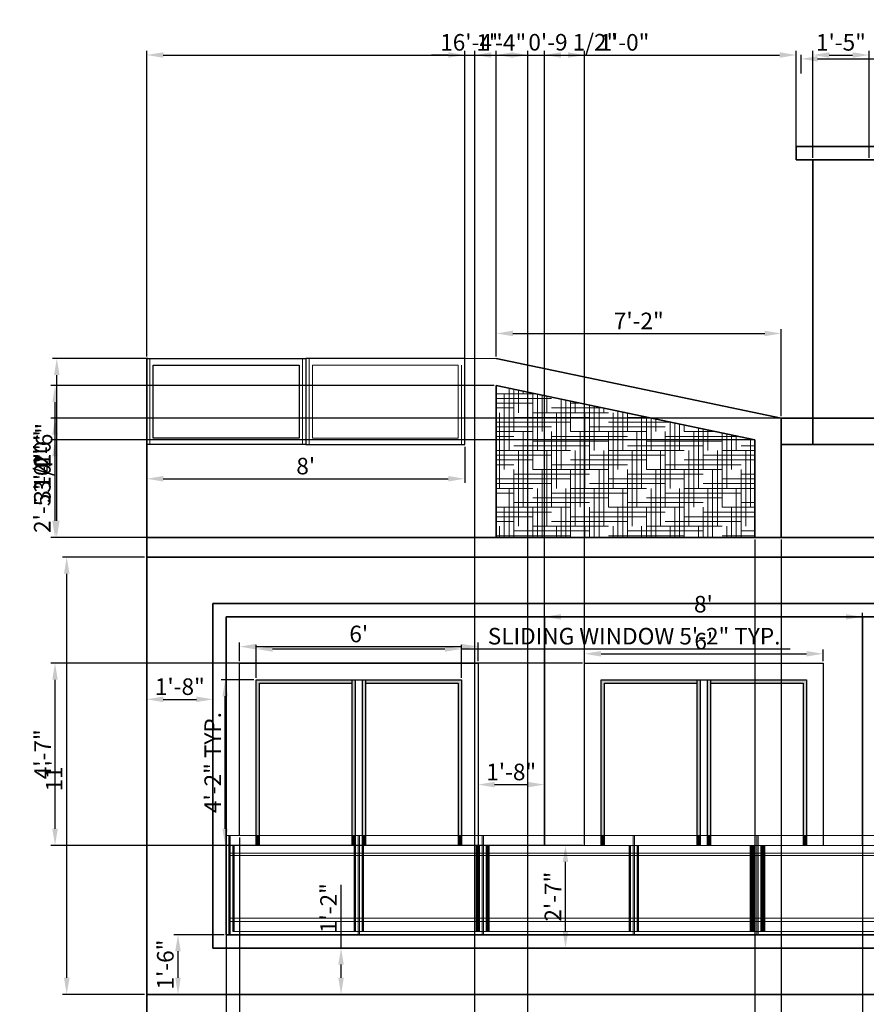
# Model space of a CAD drawing. Units: inches. Extents: x 2406 to 2953, y 1777 to 2285.
# Tile 2 of 5: x 2406 to 2661, y 1987 to 2285. Entities that reach past the tile are written whole.
import ezdxf

# ---------------------------------------------------------------- set-up
doc = ezdxf.new("R2010")
doc.units = ezdxf.units.IN
for name, color, linetype, lineweight in [('A-ANNO-DIMS', 2, 'Continuous', 18), ('A-ELEV', 7, 'Continuous', 35), ('A-ELEV-PATT', 253, 'Continuous', 13), ('A-FLOR-HRAL', 6, 'Continuous', 18), ('A-GLAZ', 4, 'Continuous', 25)]:
    doc.layers.add(name, color=color, linetype=linetype, lineweight=lineweight)
doc.styles.get("Standard").update_dxf_attribs({"font": 'arial.ttf'})
doc.dimstyles.new('ISO-25', dxfattribs={"dimtxt": 5, "dimasz": 5, "dimexe": 1.25, "dimexo": 0.625, "dimtad": 1, "dimdec": 0, "dimlunit": 3, "dimtxsty": 'Standard', "dimcen": 2.5, "dimadec": 0, "dimazin": 0, "dimtfac": 1, "dimtdec": 0, "dimtmove": 0, "dimatfit": 3, "dimfxl": 1, "dimarcsym": 0})

# ---------------------------------------------------------------- blocks, each defined once
blk = doc.blocks.new('*D7')
at = {"layer": 'A-ANNO-DIMS', "color": 0, "lineweight": -2, "transparency": 16777216}
for p, q in [((2443.21, 2122.34), (2418.45, 2122.34)), ((2419.7, 1995.34), (2419.7, 2117.34)), ((2443.21, 1990.34), (2418.45, 1990.34))]:
    blk.add_line(p, q, dxfattribs=at)
at = {"layer": 'A-ANNO-DIMS', "color": 0, "transparency": 16777216}
for points in [[(2418.87, 2117.34), (2420.53, 2117.34), (2419.7, 2122.34)], [(2418.87, 1995.34), (2420.53, 1995.34), (2419.7, 1990.34)]]:
    blk.add_solid(points, dxfattribs=at)
at = {"layer": 'Defpoints', "color": 0, "transparency": 16777216}
for p in [(2419.7, 2122.34), (2443.83, 2122.34), (2443.83, 1990.34)]:
    blk.add_point(p, dxfattribs=at)
at = {"layer": 'A-ANNO-DIMS', "color": 0, "transparency": 16777216, "insert": (2416.57, 2056.34), "char_height": 5, "attachment_point": 5, "rotation": 90}
blk.add_mtext("11'", dxfattribs=at)
blk = doc.blocks.new('*D8')
at = {"layer": 'A-ANNO-DIMS', "color": 0, "lineweight": -2, "transparency": 16777216}
for p, q in [((2444.21, 2182.34), (2415.46, 2182.34)), ((2416.71, 2133.34), (2416.71, 2177.34)), ((2443.21, 2128.34), (2415.46, 2128.34))]:
    blk.add_line(p, q, dxfattribs=at)
at = {"layer": 'A-ANNO-DIMS', "color": 0, "transparency": 16777216}
for points in [[(2415.88, 2177.34), (2417.55, 2177.34), (2416.71, 2182.34)], [(2415.88, 2133.34), (2417.55, 2133.34), (2416.71, 2128.34)]]:
    blk.add_solid(points, dxfattribs=at)
at = {"layer": 'Defpoints', "color": 0, "transparency": 16777216}
for p in [(2416.71, 2182.34), (2444.83, 2182.34), (2443.83, 2128.34)]:
    blk.add_point(p, dxfattribs=at)
at = {"layer": 'A-ANNO-DIMS', "color": 0, "transparency": 16777216, "insert": (2413.53, 2155.34), "char_height": 5, "attachment_point": 5, "rotation": 90}
blk.add_mtext('4\'-6"', dxfattribs=at)
blk = doc.blocks.new('*D9')
at = {"layer": 'A-ANNO-DIMS', "color": 0, "lineweight": -2, "transparency": 16777216}
for p, q in [((2549.33, 2182.97), (2549.33, 2191.16)), ((2554.33, 2189.91), (2630.33, 2189.91)), ((2635.33, 2164.97), (2635.33, 2191.16))]:
    blk.add_line(p, q, dxfattribs=at)
at = {"layer": 'A-ANNO-DIMS', "color": 0, "transparency": 16777216}
for points in [[(2554.33, 2190.74), (2554.33, 2189.08), (2549.33, 2189.91)], [(2630.33, 2190.74), (2630.33, 2189.08), (2635.33, 2189.91)]]:
    blk.add_solid(points, dxfattribs=at)
at = {"layer": 'Defpoints', "color": 0, "transparency": 16777216}
for p in [(2635.33, 2189.91), (2549.33, 2182.34), (2635.33, 2164.34)]:
    blk.add_point(p, dxfattribs=at)
at = {"layer": 'A-ANNO-DIMS', "color": 0, "transparency": 16777216, "insert": (2592.33, 2193.05), "char_height": 5, "attachment_point": 5}
blk.add_mtext('7\'-2"', dxfattribs=at)
blk = doc.blocks.new('*D10')
at = {"layer": 'A-ANNO-DIMS', "color": 0, "lineweight": -2, "transparency": 16777216}
for p, q in [((2641.3, 2268.37), (2641.3, 2274.08)), ((2646.3, 2272.83), (2830.3, 2272.83)), ((2835.3, 2268.37), (2835.3, 2274.08))]:
    blk.add_line(p, q, dxfattribs=at)
at = {"layer": 'A-ANNO-DIMS', "color": 0, "transparency": 16777216}
for points in [[(2646.3, 2273.66), (2646.3, 2272), (2641.3, 2272.83)], [(2830.3, 2273.66), (2830.3, 2272), (2835.3, 2272.83)]]:
    blk.add_solid(points, dxfattribs=at)
at = {"layer": 'Defpoints', "color": 0, "transparency": 16777216}
for p in [(2835.3, 2272.83), (2641.3, 2267.75), (2835.3, 2267.75)]:
    blk.add_point(p, dxfattribs=at)
at = {"layer": 'A-ANNO-DIMS', "color": 0, "transparency": 16777216, "insert": (2738.3, 2276.01), "char_height": 5, "attachment_point": 5}
blk.add_mtext('16\'-2"', dxfattribs=at)
blk = doc.blocks.new('*D13')
at = {"layer": 'A-ANNO-DIMS', "color": 0, "lineweight": -2, "transparency": 16777216}
for p, q in [((2563.83, 2097.76), (2563.83, 2105.59)), ((2659.83, 2099.01), (2659.83, 2105.59)), ((2568.83, 2104.34), (2654.83, 2104.34))]:
    blk.add_line(p, q, dxfattribs=at)
at = {"layer": 'A-ANNO-DIMS', "color": 0, "transparency": 16777216}
for points in [[(2568.83, 2105.17), (2568.83, 2103.51), (2563.83, 2104.34)], [(2654.83, 2105.17), (2654.83, 2103.51), (2659.83, 2104.34)]]:
    blk.add_solid(points, dxfattribs=at)
at = {"layer": 'Defpoints', "color": 0, "transparency": 16777216}
for p in [(2659.83, 2104.34), (2563.83, 2097.13), (2659.83, 2098.38)]:
    blk.add_point(p, dxfattribs=at)
at = {"layer": 'A-ANNO-DIMS', "color": 0, "transparency": 16777216, "insert": (2611.83, 2107.52), "char_height": 5, "attachment_point": 5}
blk.add_mtext("8'", dxfattribs=at)
blk = doc.blocks.new('*D14')
at = {"layer": 'A-ANNO-DIMS', "color": 0, "lineweight": -2, "transparency": 16777216}
for p, q in [((2575.95, 2090.97), (2575.95, 2094.44)), ((2580.95, 2093.19), (2642.95, 2093.19)), ((2647.95, 2090.97), (2647.95, 2094.44))]:
    blk.add_line(p, q, dxfattribs=at)
at = {"layer": 'A-ANNO-DIMS', "color": 0, "transparency": 16777216}
for points in [[(2580.95, 2094.02), (2580.95, 2092.35), (2575.95, 2093.19)], [(2642.95, 2094.02), (2642.95, 2092.35), (2647.95, 2093.19)]]:
    blk.add_solid(points, dxfattribs=at)
at = {"layer": 'Defpoints', "color": 0, "transparency": 16777216}
for p in [(2647.95, 2093.19), (2575.95, 2090.34), (2647.95, 2090.34)]:
    blk.add_point(p, dxfattribs=at)
at = {"layer": 'A-ANNO-DIMS', "color": 0, "transparency": 16777216, "insert": (2611.95, 2096.36), "char_height": 5, "attachment_point": 5}
blk.add_mtext("6'", dxfattribs=at)
blk = doc.blocks.new('*D22')
at = {"layer": 'A-ANNO-DIMS', "color": 0, "lineweight": -2, "transparency": 16777216}
for p, q in [((2467.21, 2008.34), (2452.04, 2008.34)), ((2453.29, 1995.34), (2453.29, 2003.34)), ((2465.03, 1990.34), (2452.04, 1990.34))]:
    blk.add_line(p, q, dxfattribs=at)
at = {"layer": 'A-ANNO-DIMS', "color": 0, "transparency": 16777216}
for points in [[(2452.45, 2003.34), (2454.12, 2003.34), (2453.29, 2008.34)], [(2452.45, 1995.34), (2454.12, 1995.34), (2453.29, 1990.34)]]:
    blk.add_solid(points, dxfattribs=at)
at = {"layer": 'Defpoints', "color": 0, "transparency": 16777216}
for p in [(2453.29, 2008.34), (2467.83, 2008.34), (2465.66, 1990.34)]:
    blk.add_point(p, dxfattribs=at)
at = {"layer": 'A-ANNO-DIMS', "color": 0, "transparency": 16777216, "insert": (2450.11, 1999.34), "char_height": 5, "attachment_point": 5, "rotation": 90}
blk.add_mtext('1\'-6"', dxfattribs=at)
blk = doc.blocks.new('*D23')
at = {"layer": 'A-ANNO-DIMS', "color": 0, "lineweight": -2, "transparency": 16777216}
for p, q in [((2502.49, 2004.34), (2502.49, 2023.41)), ((2496.37, 2004.34), (2503.74, 2004.34)), ((2502.49, 1995.34), (2502.49, 1999.34)), ((2496.37, 1990.34), (2503.74, 1990.34))]:
    blk.add_line(p, q, dxfattribs=at)
at = {"layer": 'A-ANNO-DIMS', "color": 0, "transparency": 16777216}
for points in [[(2501.66, 1999.34), (2503.32, 1999.34), (2502.49, 2004.34)], [(2501.66, 1995.34), (2503.32, 1995.34), (2502.49, 1990.34)]]:
    blk.add_solid(points, dxfattribs=at)
at = {"layer": 'Defpoints', "color": 0, "transparency": 16777216}
for p in [(2495.74, 2004.34), (2502.49, 2004.34), (2495.74, 1990.34)]:
    blk.add_point(p, dxfattribs=at)
at = {"layer": 'A-ANNO-DIMS', "color": 0, "transparency": 16777216, "insert": (2499.36, 2016.38), "char_height": 5, "attachment_point": 5, "rotation": 90}
blk.add_mtext('1\'-2"', dxfattribs=at)
blk = doc.blocks.new('*D24')
at = {"layer": 'A-ANNO-DIMS', "color": 0, "lineweight": -2, "transparency": 16777216}
for p, q in [((2443.83, 2067.83), (2443.83, 2080.68)), ((2448.83, 2079.43), (2458.83, 2079.43)), ((2463.83, 2067.83), (2463.83, 2080.68))]:
    blk.add_line(p, q, dxfattribs=at)
at = {"layer": 'A-ANNO-DIMS', "color": 0, "transparency": 16777216}
for points in [[(2448.83, 2080.27), (2448.83, 2078.6), (2443.83, 2079.43)], [(2458.83, 2080.27), (2458.83, 2078.6), (2463.83, 2079.43)]]:
    blk.add_solid(points, dxfattribs=at)
at = {"layer": 'Defpoints', "color": 0, "transparency": 16777216}
for p in [(2463.83, 2079.43), (2443.83, 2067.21), (2463.83, 2067.21)]:
    blk.add_point(p, dxfattribs=at)
at = {"layer": 'A-ANNO-DIMS', "color": 0, "transparency": 16777216, "insert": (2453.83, 2082.61), "char_height": 5, "attachment_point": 5}
blk.add_mtext('1\'-8"', dxfattribs=at)
blk = doc.blocks.new('*D33')
at = {"layer": 'A-ANNO-DIMS', "color": 0, "lineweight": -2, "transparency": 16777216}
for p, q in [((2575.33, 2035.34), (2568.96, 2035.34)), ((2570.21, 2009.34), (2570.21, 2030.34)), ((2574.25, 2004.34), (2568.96, 2004.34))]:
    blk.add_line(p, q, dxfattribs=at)
at = {"layer": 'A-ANNO-DIMS', "color": 0, "transparency": 16777216}
for points in [[(2569.38, 2030.34), (2571.04, 2030.34), (2570.21, 2035.34)], [(2569.38, 2009.34), (2571.04, 2009.34), (2570.21, 2004.34)]]:
    blk.add_solid(points, dxfattribs=at)
at = {"layer": 'Defpoints', "color": 0, "transparency": 16777216}
for p in [(2570.21, 2035.34), (2575.95, 2035.34), (2574.87, 2004.34)]:
    blk.add_point(p, dxfattribs=at)
at = {"layer": 'A-ANNO-DIMS', "color": 0, "transparency": 16777216, "insert": (2567.07, 2019.84), "char_height": 5, "attachment_point": 5, "rotation": 90}
blk.add_mtext('2\'-7"', dxfattribs=at)
blk = doc.blocks.new('*D34')
at = {"layer": 'A-ANNO-DIMS', "color": 0, "lineweight": -2, "transparency": 16777216}
for p, q in [((2471.83, 2090.97), (2471.83, 2096.59)), ((2543.83, 2090.97), (2543.83, 2096.59)), ((2476.83, 2095.34), (2538.83, 2095.34))]:
    blk.add_line(p, q, dxfattribs=at)
at = {"layer": 'A-ANNO-DIMS', "color": 0, "transparency": 16777216}
for points in [[(2476.83, 2096.18), (2476.83, 2094.51), (2471.83, 2095.34)], [(2538.83, 2096.18), (2538.83, 2094.51), (2543.83, 2095.34)]]:
    blk.add_solid(points, dxfattribs=at)
at = {"layer": 'Defpoints', "color": 0, "transparency": 16777216}
for p in [(2543.83, 2095.34), (2471.83, 2090.34), (2543.83, 2090.34)]:
    blk.add_point(p, dxfattribs=at)
at = {"layer": 'A-ANNO-DIMS', "color": 0, "transparency": 16777216, "insert": (2507.83, 2098.52), "char_height": 5, "attachment_point": 5}
blk.add_mtext("6'", dxfattribs=at)
blk = doc.blocks.new('*D35')
at = {"layer": 'A-ANNO-DIMS', "color": 0, "lineweight": -2, "transparency": 16777216}
for p, q in [((2543.83, 2062.22), (2543.83, 2052.43)), ((2563.83, 2062.22), (2563.83, 2052.43)), ((2548.83, 2053.68), (2558.83, 2053.68))]:
    blk.add_line(p, q, dxfattribs=at)
at = {"layer": 'A-ANNO-DIMS', "color": 0, "transparency": 16777216}
for points in [[(2548.83, 2054.51), (2548.83, 2052.84), (2543.83, 2053.68)], [(2558.83, 2054.51), (2558.83, 2052.84), (2563.83, 2053.68)]]:
    blk.add_solid(points, dxfattribs=at)
at = {"layer": 'Defpoints', "color": 0, "transparency": 16777216}
for p in [(2543.83, 2062.84), (2563.83, 2062.84), (2563.83, 2053.68)]:
    blk.add_point(p, dxfattribs=at)
at = {"layer": 'A-ANNO-DIMS', "color": 0, "transparency": 16777216, "insert": (2553.83, 2056.85), "char_height": 5, "attachment_point": 5}
blk.add_mtext('1\'-8"', dxfattribs=at)
blk = doc.blocks.new('*D36')
at = {"layer": 'A-ANNO-DIMS', "color": 0, "lineweight": -2, "transparency": 16777216}
for p, q in [((2443.83, 2155.72), (2443.83, 2144.78)), ((2539.83, 2155.72), (2539.83, 2144.78)), ((2448.83, 2146.03), (2534.83, 2146.03))]:
    blk.add_line(p, q, dxfattribs=at)
at = {"layer": 'A-ANNO-DIMS', "color": 0, "transparency": 16777216}
for points in [[(2448.83, 2146.87), (2448.83, 2145.2), (2443.83, 2146.03)], [(2534.83, 2146.87), (2534.83, 2145.2), (2539.83, 2146.03)]]:
    blk.add_solid(points, dxfattribs=at)
at = {"layer": 'Defpoints', "color": 0, "transparency": 16777216}
for p in [(2443.83, 2156.34), (2539.83, 2156.34), (2539.83, 2146.03)]:
    blk.add_point(p, dxfattribs=at)
at = {"layer": 'A-ANNO-DIMS', "color": 0, "transparency": 16777216, "insert": (2491.83, 2149.21), "char_height": 5, "attachment_point": 5}
blk.add_mtext("8'", dxfattribs=at)
blk = doc.blocks.new('WIN-SLIDING-1500')
for p, q in [((0, 50), (62, 50)), ((0, 0), (0, 50)), ((1, 0), (1, 49)), ((1, 49), (29, 49)), ((29, 0), (29, 50)), ((30, 0), (30, 50)), ((32, 50), (32, 0)), ((33, 50), (33, 0)), ((33, 49), (61, 49)), ((61, 49), (61, 0)), ((62, 50), (62, 0))]:
    blk.add_line(p, q)
blk = doc.blocks.new('*D41')
at = {"layer": 'A-ANNO-DIMS', "color": 0, "lineweight": -2, "transparency": 16777216}
for p, q in [((2476.83, 2085.97), (2476.83, 2095.89)), ((2481.83, 2094.64), (2533.83, 2094.64)), ((2538.83, 2085.97), (2538.83, 2095.89)), ((2538.83, 2094.64), (2638.01, 2094.64))]:
    blk.add_line(p, q, dxfattribs=at)
at = {"layer": 'A-ANNO-DIMS', "color": 0, "transparency": 16777216}
for points in [[(2481.83, 2095.47), (2481.83, 2093.81), (2476.83, 2094.64)], [(2533.83, 2095.47), (2533.83, 2093.81), (2538.83, 2094.64)]]:
    blk.add_solid(points, dxfattribs=at)
at = {"layer": 'Defpoints', "color": 0, "transparency": 16777216}
for p in [(2538.83, 2094.64), (2476.83, 2085.34), (2538.83, 2085.34)]:
    blk.add_point(p, dxfattribs=at)
at = {"layer": 'A-ANNO-DIMS', "color": 0, "transparency": 16777216, "insert": (2590.92, 2097.85), "char_height": 5, "attachment_point": 5}
blk.add_mtext('SLIDING WINDOW 5\'-2" TYP.', dxfattribs=at)
blk = doc.blocks.new('*D42')
at = {"layer": 'A-ANNO-DIMS', "color": 0, "lineweight": -2, "transparency": 16777216}
for p, q in [((2476.21, 2085.34), (2466.28, 2085.34)), ((2467.53, 2040.34), (2467.53, 2080.34)), ((2476.21, 2035.34), (2466.28, 2035.34))]:
    blk.add_line(p, q, dxfattribs=at)
at = {"layer": 'A-ANNO-DIMS', "color": 0, "transparency": 16777216}
for points in [[(2466.7, 2080.34), (2468.37, 2080.34), (2467.53, 2085.34)], [(2466.7, 2040.34), (2468.37, 2040.34), (2467.53, 2035.34)]]:
    blk.add_solid(points, dxfattribs=at)
at = {"layer": 'Defpoints', "color": 0, "transparency": 16777216}
for p in [(2467.53, 2085.34), (2476.83, 2085.34), (2476.83, 2035.34)]:
    blk.add_point(p, dxfattribs=at)
at = {"layer": 'A-ANNO-DIMS', "color": 0, "transparency": 16777216, "insert": (2464.4, 2060.34), "char_height": 5, "attachment_point": 5, "rotation": 90}
blk.add_mtext('4\'-2" TYP.', dxfattribs=at)
blk = doc.blocks.new('*D45')
at = {"layer": 'A-ANNO-DIMS', "color": 0, "lineweight": -2, "transparency": 16777216}
for p, q in [((2673.85, 1912.9), (2673.85, 2012.41)), ((2681.47, 1912.9), (2672.6, 1912.9)), ((2673.85, 1862.91), (2673.85, 1907.9)), ((2681.47, 1857.91), (2672.6, 1857.91))]:
    blk.add_line(p, q, dxfattribs=at)
at = {"layer": 'A-ANNO-DIMS', "color": 0, "transparency": 16777216}
for points in [[(2673.01, 1907.9), (2674.68, 1907.9), (2673.85, 1912.9)], [(2673.01, 1862.91), (2674.68, 1862.91), (2673.85, 1857.91)]]:
    blk.add_solid(points, dxfattribs=at)
at = {"layer": 'Defpoints', "color": 0, "transparency": 16777216}
for p in [(2673.85, 1912.9), (2682.1, 1912.9), (2682.1, 1857.91)]:
    blk.add_point(p, dxfattribs=at)
at = {"layer": 'A-ANNO-DIMS', "color": 0, "transparency": 16777216, "insert": (2670.64, 1965.16), "char_height": 5, "attachment_point": 5, "rotation": 90}
blk.add_mtext('GATE ORNAMENT 4\'-7" TYP.', dxfattribs=at)
blk = doc.blocks.new('*D47')
at = {"layer": 'A-ANNO-DIMS', "color": 0, "lineweight": -2, "transparency": 16777216}
for p, q in [((2542.83, 1957.97), (2542.83, 2275.24)), ((2558.83, 1957.97), (2558.83, 2275.24)), ((2547.83, 2273.99), (2553.83, 2273.99))]:
    blk.add_line(p, q, dxfattribs=at)
at = {"layer": 'A-ANNO-DIMS', "color": 0, "transparency": 16777216}
for points in [[(2547.83, 2274.82), (2547.83, 2273.16), (2542.83, 2273.99)], [(2553.83, 2274.82), (2553.83, 2273.16), (2558.83, 2273.99)]]:
    blk.add_solid(points, dxfattribs=at)
at = {"layer": 'Defpoints', "color": 0, "transparency": 16777216}
for p in [(2558.83, 2273.99), (2542.83, 1957.34), (2558.83, 1957.34)]:
    blk.add_point(p, dxfattribs=at)
at = {"layer": 'A-ANNO-DIMS', "color": 0, "transparency": 16777216, "insert": (2550.83, 2277.13), "char_height": 5, "attachment_point": 5}
blk.add_mtext('1\'-4"', dxfattribs=at)
blk = doc.blocks.new('*D62')
at = {"layer": 'A-ANNO-DIMS', "color": 0, "lineweight": -2, "transparency": 16777216}
for p, q in [((2467.83, 2037.72), (2467.83, 1793.44)), ((2471.83, 2037.72), (2471.83, 1793.44)), ((2462.83, 1794.69), (2457.83, 1794.69)), ((2467.83, 1794.69), (2471.83, 1794.69)), ((2476.83, 1794.69), (2496.37, 1794.69))]:
    blk.add_line(p, q, dxfattribs=at)
at = {"layer": 'A-ANNO-DIMS', "color": 0, "transparency": 16777216}
for points in [[(2462.83, 1795.52), (2462.83, 1793.86), (2467.83, 1794.69)], [(2476.83, 1795.52), (2476.83, 1793.86), (2471.83, 1794.69)]]:
    blk.add_solid(points, dxfattribs=at)
at = {"layer": 'Defpoints', "color": 0, "transparency": 16777216}
for p in [(2467.83, 2038.34), (2471.83, 2038.34), (2471.83, 1794.69)]:
    blk.add_point(p, dxfattribs=at)
at = {"layer": 'A-ANNO-DIMS', "color": 0, "transparency": 16777216, "insert": (2489.1, 1797.87), "char_height": 5, "attachment_point": 5}
blk.add_mtext('0\'-4"', dxfattribs=at)
blk = doc.blocks.new('*D63')
at = {"layer": 'A-ANNO-DIMS', "color": 0, "lineweight": -2, "transparency": 16777216}
for p, q in [((2563.83, 2035.97), (2563.83, 2275.24)), ((2575.95, 2035.97), (2575.95, 2275.24)), ((2568.83, 2273.99), (2570.95, 2273.99)), ((2575.95, 2273.99), (2595.02, 2273.99))]:
    blk.add_line(p, q, dxfattribs=at)
at = {"layer": 'A-ANNO-DIMS', "color": 0, "transparency": 16777216}
for points in [[(2568.83, 2274.82), (2568.83, 2273.16), (2563.83, 2273.99)], [(2570.95, 2274.82), (2570.95, 2273.16), (2575.95, 2273.99)]]:
    blk.add_solid(points, dxfattribs=at)
at = {"layer": 'Defpoints', "color": 0, "transparency": 16777216}
for p in [(2575.95, 2273.99), (2563.83, 2035.34), (2575.95, 2035.34)]:
    blk.add_point(p, dxfattribs=at)
at = {"layer": 'A-ANNO-DIMS', "color": 0, "transparency": 16777216, "insert": (2587.99, 2277.17), "char_height": 5, "attachment_point": 5}
blk.add_mtext('1\'-0"', dxfattribs=at)
blk = doc.blocks.new('*D64')
at = {"layer": 'A-ANNO-DIMS', "color": 0, "lineweight": -2, "transparency": 16777216}
for p, q in [((2659.83, 2103.72), (2659.83, 1793.44)), ((2671.83, 2089.72), (2671.83, 1793.44)), ((2664.83, 1794.69), (2666.83, 1794.69)), ((2671.83, 1794.69), (2690.9, 1794.69))]:
    blk.add_line(p, q, dxfattribs=at)
at = {"layer": 'A-ANNO-DIMS', "color": 0, "transparency": 16777216}
for points in [[(2664.83, 1795.52), (2664.83, 1793.86), (2659.83, 1794.69)], [(2666.83, 1795.52), (2666.83, 1793.86), (2671.83, 1794.69)]]:
    blk.add_solid(points, dxfattribs=at)
at = {"layer": 'Defpoints', "color": 0, "transparency": 16777216}
for p in [(2659.83, 2104.34), (2671.83, 2090.34), (2671.83, 1794.69)]:
    blk.add_point(p, dxfattribs=at)
at = {"layer": 'A-ANNO-DIMS', "color": 0, "transparency": 16777216, "insert": (2683.87, 1797.87), "char_height": 5, "attachment_point": 5}
blk.add_mtext('1\'-0"', dxfattribs=at)
blk = doc.blocks.new('*D66')
at = {"layer": 'A-ANNO-DIMS', "color": 0, "lineweight": -2, "transparency": 16777216}
for p, q in [((2575.33, 2090.34), (2414.93, 2090.34)), ((2416.18, 2040.34), (2416.18, 2085.34)), ((2575.33, 2035.34), (2414.93, 2035.34))]:
    blk.add_line(p, q, dxfattribs=at)
at = {"layer": 'A-ANNO-DIMS', "color": 0, "transparency": 16777216}
for points in [[(2415.35, 2085.34), (2417.02, 2085.34), (2416.18, 2090.34)], [(2415.35, 2040.34), (2417.02, 2040.34), (2416.18, 2035.34)]]:
    blk.add_solid(points, dxfattribs=at)
at = {"layer": 'Defpoints', "color": 0, "transparency": 16777216}
for p in [(2416.18, 2090.34), (2575.95, 2090.34), (2575.95, 2035.34)]:
    blk.add_point(p, dxfattribs=at)
at = {"layer": 'A-ANNO-DIMS', "color": 0, "transparency": 16777216, "insert": (2413.06, 2062.84), "char_height": 5, "attachment_point": 5, "rotation": 90}
blk.add_mtext('4\'-7"', dxfattribs=at)
blk = doc.blocks.new('*D73')
at = {"layer": 'A-ANNO-DIMS', "color": 0, "lineweight": -2, "transparency": 16777216}
for p, q in [((2634.71, 2164.34), (2414.93, 2164.34)), ((2416.18, 2133.34), (2416.18, 2159.34)), ((2634.71, 2128.34), (2414.93, 2128.34))]:
    blk.add_line(p, q, dxfattribs=at)
at = {"layer": 'A-ANNO-DIMS', "color": 0, "transparency": 16777216}
for points in [[(2415.35, 2159.34), (2417.02, 2159.34), (2416.18, 2164.34)], [(2415.35, 2133.34), (2417.02, 2133.34), (2416.18, 2128.34)]]:
    blk.add_solid(points, dxfattribs=at)
at = {"layer": 'Defpoints', "color": 0, "transparency": 16777216}
for p in [(2416.18, 2164.34), (2635.33, 2164.34), (2635.33, 2128.34)]:
    blk.add_point(p, dxfattribs=at)
at = {"layer": 'A-ANNO-DIMS', "color": 0, "transparency": 16777216, "insert": (2413, 2146.34), "char_height": 5, "attachment_point": 5, "rotation": 90}
blk.add_mtext('3\'-0"', dxfattribs=at)
blk = doc.blocks.new('*D74')
at = {"layer": 'A-ANNO-DIMS', "color": 0, "lineweight": -2, "transparency": 16777216}
for p, q in [((2548.71, 2174.17), (2414.93, 2174.17)), ((2416.18, 2133.34), (2416.18, 2169.17)), ((2548.71, 2128.34), (2414.93, 2128.34))]:
    blk.add_line(p, q, dxfattribs=at)
at = {"layer": 'A-ANNO-DIMS', "color": 0, "transparency": 16777216}
for points in [[(2415.35, 2169.17), (2417.02, 2169.17), (2416.18, 2174.17)], [(2415.35, 2133.34), (2417.02, 2133.34), (2416.18, 2128.34)]]:
    blk.add_solid(points, dxfattribs=at)
at = {"layer": 'Defpoints', "color": 0, "transparency": 16777216}
for p in [(2416.18, 2174.17), (2549.33, 2174.17), (2549.33, 2128.34)]:
    blk.add_point(p, dxfattribs=at)
at = {"layer": 'A-ANNO-DIMS', "color": 0, "transparency": 16777216, "insert": (2413, 2151.25), "char_height": 5, "attachment_point": 5, "rotation": 90}
blk.add_mtext('3\'-10"', dxfattribs=at)
blk = doc.blocks.new('*D75')
at = {"layer": 'A-ANNO-DIMS', "color": 0, "lineweight": -2, "transparency": 16777216}
for p, q in [((2626.71, 2157.84), (2414.93, 2157.84)), ((2416.18, 2133.34), (2416.18, 2152.84)), ((2626.71, 2128.34), (2414.93, 2128.34))]:
    blk.add_line(p, q, dxfattribs=at)
at = {"layer": 'A-ANNO-DIMS', "color": 0, "transparency": 16777216}
for points in [[(2415.35, 2152.84), (2417.02, 2152.84), (2416.18, 2157.84)], [(2415.35, 2133.34), (2417.02, 2133.34), (2416.18, 2128.34)]]:
    blk.add_solid(points, dxfattribs=at)
at = {"layer": 'Defpoints', "color": 0, "transparency": 16777216}
for p in [(2416.18, 2157.84), (2627.33, 2157.84), (2627.33, 2128.34)]:
    blk.add_point(p, dxfattribs=at)
at = {"layer": 'A-ANNO-DIMS', "color": 0, "transparency": 16777216, "insert": (2412.97, 2143.09), "char_height": 5, "attachment_point": 5, "rotation": 90}
blk.add_mtext('2\'-5 1/2"', dxfattribs=at)
blk = doc.blocks.new('*D76')
at = {"layer": 'A-ANNO-DIMS', "color": 0, "lineweight": -2, "transparency": 16777216}
for p, q in [((2627.33, 2127.72), (2627.33, 1793.44)), ((2635.33, 2127.72), (2635.33, 1793.44)), ((2622.33, 1794.69), (2617.33, 1794.69)), ((2627.33, 1794.69), (2635.33, 1794.69)), ((2640.33, 1794.69), (2659.87, 1794.69))]:
    blk.add_line(p, q, dxfattribs=at)
at = {"layer": 'A-ANNO-DIMS', "color": 0, "transparency": 16777216}
for points in [[(2622.33, 1795.52), (2622.33, 1793.86), (2627.33, 1794.69)], [(2640.33, 1795.52), (2640.33, 1793.86), (2635.33, 1794.69)]]:
    blk.add_solid(points, dxfattribs=at)
at = {"layer": 'Defpoints', "color": 0, "transparency": 16777216}
for p in [(2627.33, 2128.34), (2635.33, 2128.34), (2635.33, 1794.69)]:
    blk.add_point(p, dxfattribs=at)
at = {"layer": 'A-ANNO-DIMS', "color": 0, "transparency": 16777216, "insert": (2652.6, 1797.87), "char_height": 5, "attachment_point": 5}
blk.add_mtext('0\'-8"', dxfattribs=at)
blk = doc.blocks.new('*D77')
at = {"layer": 'A-ANNO-DIMS', "color": 0, "lineweight": -2, "transparency": 16777216}
for p, q in [((2539.83, 2156.97), (2539.83, 2275.24)), ((2549.33, 2182.97), (2549.33, 2275.24)), ((2534.83, 2273.99), (2529.83, 2273.99)), ((2539.83, 2273.99), (2549.33, 2273.99)), ((2554.33, 2273.99), (2585.53, 2273.99))]:
    blk.add_line(p, q, dxfattribs=at)
at = {"layer": 'A-ANNO-DIMS', "color": 0, "transparency": 16777216}
for points in [[(2534.83, 2274.82), (2534.83, 2273.16), (2539.83, 2273.99)], [(2554.33, 2274.82), (2554.33, 2273.16), (2549.33, 2273.99)]]:
    blk.add_solid(points, dxfattribs=at)
at = {"layer": 'Defpoints', "color": 0, "transparency": 16777216}
for p in [(2549.33, 2273.99), (2549.33, 2182.34), (2539.83, 2156.34)]:
    blk.add_point(p, dxfattribs=at)
at = {"layer": 'A-ANNO-DIMS', "color": 0, "transparency": 16777216, "insert": (2572.43, 2277.2), "char_height": 5, "attachment_point": 5}
blk.add_mtext('0\'-9 1/2"', dxfattribs=at)
blk = doc.blocks.new('*D78')
at = {"layer": 'A-ANNO-DIMS', "color": 0, "lineweight": -2, "transparency": 16777216}
for p, q in [((2443.83, 2182.97), (2443.83, 2275.24)), ((2639.83, 2242.97), (2639.83, 2275.24)), ((2448.83, 2273.99), (2634.83, 2273.99))]:
    blk.add_line(p, q, dxfattribs=at)
at = {"layer": 'A-ANNO-DIMS', "color": 0, "transparency": 16777216}
for points in [[(2448.83, 2274.82), (2448.83, 2273.16), (2443.83, 2273.99)], [(2634.83, 2274.82), (2634.83, 2273.16), (2639.83, 2273.99)]]:
    blk.add_solid(points, dxfattribs=at)
at = {"layer": 'Defpoints', "color": 0, "transparency": 16777216}
for p in [(2639.83, 2273.99), (2639.83, 2242.34), (2443.83, 2182.34)]:
    blk.add_point(p, dxfattribs=at)
at = {"layer": 'A-ANNO-DIMS', "color": 0, "transparency": 16777216, "insert": (2541.83, 2277.17), "char_height": 5, "attachment_point": 5}
blk.add_mtext('16\'-4"', dxfattribs=at)
blk = doc.blocks.new('*D79')
at = {"layer": 'A-ANNO-DIMS', "color": 0, "lineweight": -2, "transparency": 16777216}
for p, q in [((2861.48, 2251.34), (2861.48, 2270.88)), ((2640.46, 2246.34), (2862.73, 2246.34)), ((2861.48, 2242.34), (2861.48, 2246.34)), ((2640.46, 2242.34), (2862.73, 2242.34)), ((2861.48, 2237.34), (2861.48, 2232.34))]:
    blk.add_line(p, q, dxfattribs=at)
at = {"layer": 'A-ANNO-DIMS', "color": 0, "transparency": 16777216}
for points in [[(2860.65, 2251.34), (2862.32, 2251.34), (2861.48, 2246.34)], [(2860.65, 2237.34), (2862.32, 2237.34), (2861.48, 2242.34)]]:
    blk.add_solid(points, dxfattribs=at)
at = {"layer": 'Defpoints', "color": 0, "transparency": 16777216}
for p in [(2639.83, 2246.34), (2861.48, 2246.34), (2639.83, 2242.34)]:
    blk.add_point(p, dxfattribs=at)
at = {"layer": 'A-ANNO-DIMS', "color": 0, "transparency": 16777216, "insert": (2858.31, 2263.61), "char_height": 5, "attachment_point": 5, "rotation": 90}
blk.add_mtext('0\'-4"', dxfattribs=at)
blk = doc.blocks.new('*D80')
at = {"layer": 'A-ANNO-DIMS', "color": 0, "lineweight": -2, "transparency": 16777216}
for p, q in [((2644.83, 2242.97), (2644.83, 2275.24)), ((2661.83, 2242.97), (2661.83, 2275.24)), ((2649.83, 2273.99), (2656.83, 2273.99))]:
    blk.add_line(p, q, dxfattribs=at)
at = {"layer": 'A-ANNO-DIMS', "color": 0, "transparency": 16777216}
for points in [[(2649.83, 2274.82), (2649.83, 2273.16), (2644.83, 2273.99)], [(2656.83, 2274.82), (2656.83, 2273.16), (2661.83, 2273.99)]]:
    blk.add_solid(points, dxfattribs=at)
at = {"layer": 'Defpoints', "color": 0, "transparency": 16777216}
for p in [(2661.83, 2273.99), (2644.83, 2242.34), (2661.83, 2242.34)]:
    blk.add_point(p, dxfattribs=at)
at = {"layer": 'A-ANNO-DIMS', "color": 0, "transparency": 16777216, "insert": (2653.33, 2277.17), "char_height": 5, "attachment_point": 5}
blk.add_mtext('1\'-5"', dxfattribs=at)

msp = doc.modelspace()

# ---------------------------------------------------------------- hatches: boundary and pattern name
at = {"layer": 'A-ELEV-PATT'}
h = msp.add_hatch(dxfattribs=at)
h.set_pattern_fill('HOUND', color=256, scale=0.9)
h.paths.add_polyline_path([(2627.33, 2157.84), (2549.33, 2174.17), (2549.33, 2128.34), (2627.33, 2128.34)])
h = msp.add_hatch(color=256, dxfattribs=at)
h.dxf.hatch_style = 1
h.paths.add_polyline_path([(2476.83, 2038.34), (2477.83, 2038.34), (2477.83, 2084.34), (2505.83, 2084.34), (2505.83, 2085.34), (2476.83, 2085.34)])
h = msp.add_hatch(color=256, dxfattribs=at)
h.dxf.hatch_style = 1
h.paths.add_polyline_path([(2506.83, 2085.34), (2505.83, 2085.34), (2505.83, 2038.34), (2506.83, 2038.34)])
h = msp.add_hatch(color=256, dxfattribs=at)
h.dxf.hatch_style = 1
h.paths.add_polyline_path([(2509.83, 2085.34), (2508.83, 2085.34), (2508.83, 2038.34), (2509.83, 2038.34)])
h = msp.add_hatch(color=256, dxfattribs=at)
h.dxf.hatch_style = 1
h.paths.add_polyline_path([(2509.83, 2085.34), (2509.83, 2084.34), (2537.83, 2084.34), (2537.83, 2038.34), (2538.83, 2038.34), (2538.83, 2085.34)])
h = msp.add_hatch(color=256, dxfattribs=at)
h.dxf.hatch_style = 1
h.paths.add_polyline_path([(2609.95, 2084.34), (2609.95, 2085.34), (2580.95, 2085.34), (2580.95, 2038.34), (2581.95, 2038.34), (2581.95, 2084.34)])
h = msp.add_hatch(color=256, dxfattribs=at)
h.dxf.hatch_style = 1
h.paths.add_polyline_path([(2609.95, 2038.34), (2610.95, 2038.34), (2610.95, 2085.34), (2609.95, 2085.34)])
h = msp.add_hatch(color=256, dxfattribs=at)
h.dxf.hatch_style = 1
h.paths.add_polyline_path([(2612.95, 2038.34), (2613.95, 2038.34), (2613.95, 2085.34), (2612.95, 2085.34)])
h = msp.add_hatch(color=256, dxfattribs=at)
h.dxf.hatch_style = 1
h.paths.add_polyline_path([(2641.95, 2084.34), (2641.95, 2038.34), (2642.95, 2038.34), (2642.95, 2085.34), (2613.95, 2085.34), (2613.95, 2084.34)])
h = msp.add_hatch(color=256, dxfattribs=at)
h.dxf.hatch_style = 1
h.paths.add_polyline_path([(2477.83, 2038.34), (2476.83, 2038.34), (2476.83, 2035.34), (2477.83, 2035.34)])
h = msp.add_hatch(color=256, dxfattribs=at)
h.dxf.hatch_style = 1
h.paths.add_polyline_path([(2505.83, 2035.34), (2506.83, 2035.34), (2506.83, 2038.34), (2505.83, 2038.34)])
h = msp.add_hatch(color=256, dxfattribs=at)
h.dxf.hatch_style = 1
h.paths.add_polyline_path([(2509.83, 2038.34), (2508.83, 2038.34), (2508.83, 2035.34), (2509.83, 2035.34)])
h = msp.add_hatch(color=256, dxfattribs=at)
h.dxf.hatch_style = 1
h.paths.add_polyline_path([(2538.83, 2038.34), (2537.83, 2038.34), (2537.83, 2035.34), (2538.83, 2035.34)])
h = msp.add_hatch(color=256, dxfattribs=at)
h.dxf.hatch_style = 1
h.paths.add_polyline_path([(2581.95, 2038.34), (2580.95, 2038.34), (2580.95, 2035.34), (2581.95, 2035.34)])
h = msp.add_hatch(color=256, dxfattribs=at)
h.dxf.hatch_style = 1
h.paths.add_polyline_path([(2609.95, 2035.34), (2610.95, 2035.34), (2610.95, 2038.34), (2609.95, 2038.34)])
h = msp.add_hatch(color=256, dxfattribs=at)
h.dxf.hatch_style = 1
h.paths.add_polyline_path([(2613.95, 2038.34), (2612.95, 2038.34), (2612.95, 2035.34), (2613.95, 2035.34)])
h = msp.add_hatch(color=256, dxfattribs=at)
h.dxf.hatch_style = 1
h.paths.add_polyline_path([(2641.95, 2035.34), (2642.95, 2035.34), (2642.95, 2038.34), (2641.95, 2038.34)])

# ---------------------------------------------------------------- linework, layer by layer
at = {"layer": 'A-ELEV'}
for p, q in [((2639.83, 2242.34), (2639.83, 2246.34)), ((2833.83, 2246.34), (2639.83, 2246.34)), ((2833.83, 2242.34), (2639.83, 2242.34)), ((2644.83, 2156.34), (2644.83, 2242.34)), ((2443.83, 2182.34), (2443.83, 1822.34)), ((2549.33, 2182.34), (2635.33, 2164.34)), ((2549.33, 2174.17), (2549.33, 2128.34)), ((2549.33, 2174.17), (2627.33, 2157.84)), ((2635.33, 2164.34), (2635.33, 2128.34)), ((2635.33, 2164.34), (2827.83, 2164.34)), ((2627.33, 2157.84), (2627.33, 2128.34)), ((2635.33, 2156.34), (2808.31, 2156.34)), ((2443.83, 2128.34), (2827.83, 2128.34)), ((2443.83, 2122.34), (2827.83, 2122.34)), ((2443.83, 2122.34), (2443.83, 1990.34)), ((2463.83, 2108.34), (2463.83, 2004.34)), ((2463.83, 2108.34), (2827.83, 2108.34)), ((2467.83, 2104.34), (2802.83, 2104.34)), ((2467.83, 2104.34), (2467.83, 2008.34)), ((2467.83, 2038.34), (2467.83, 2104.34)), ((2563.83, 2035.34), (2563.83, 2104.34)), ((2659.83, 2035.34), (2659.83, 2104.34)), ((2467.83, 2008.34), (2767.46, 2008.34)), ((2463.83, 2004.34), (2827.83, 2004.34)), ((2443.83, 1990.34), (2827.83, 1990.34))]:
    msp.add_line(p, q, dxfattribs=at)
at = {"layer": 'A-FLOR-HRAL'}
for p, q in [((2443.83, 2182.34), (2539.83, 2182.34)), ((2443.83, 2152.34), (2443.83, 2182.34)), ((2444.83, 2156.34), (2444.83, 2182.34)), ((2490.83, 2156.34), (2490.83, 2182.34)), ((2491.83, 2156.34), (2491.83, 2182.34)), ((2492.83, 2182.34), (2492.83, 2156.34)), ((2539.83, 2156.34), (2539.83, 2182.34)), ((2539.83, 2182.34), (2549.33, 2182.34)), ((2445.83, 2158.34), (2445.83, 2180.34)), ((2489.83, 2158.34), (2489.83, 2180.34)), ((2537.83, 2180.34), (2493.83, 2180.34)), ((2493.83, 2180.34), (2493.83, 2158.34)), ((2537.83, 2158.34), (2537.83, 2180.34)), ((2538.83, 2156.34), (2538.83, 2180.34)), ((2443.83, 2156.34), (2539.83, 2156.34)), ((2493.83, 2158.34), (2537.83, 2158.34)), ((2467.83, 2038.34), (2695.83, 2038.34)), ((2468.63, 2038.34), (2468.63, 2008.34)), ((2468.83, 2035.34), (2468.83, 2038.34)), ((2469.03, 2038.34), (2469.03, 2008.34)), ((2471.83, 2038.34), (2543.83, 2038.34)), ((2507.63, 2038.34), (2507.63, 2008.34)), ((2508.03, 2038.34), (2508.03, 2008.34)), ((2543.83, 2038.34), (2543.83, 2038.34)), ((2545.03, 2038.34), (2545.03, 2008.34)), ((2545.43, 2038.34), (2545.43, 2008.34)), ((2590.6, 2038.34), (2590.6, 2008.34)), ((2591, 2038.34), (2591, 2008.34)), ((2627.93, 2038.34), (2627.93, 2008.34)), ((2628.33, 2038.34), (2628.33, 2008.34)), ((2468.83, 2035.34), (2468.83, 2008.34)), ((2469.83, 2035.34), (2692.83, 2035.34)), ((2469.83, 2035.34), (2469.83, 2009.34)), ((2470.03, 2035.34), (2470.03, 2009.34)), ((2470.23, 2035.34), (2470.23, 2009.34)), ((2506.43, 2035.34), (2506.43, 2009.34)), ((2506.63, 2035.34), (2506.63, 2009.34)), ((2506.83, 2035.34), (2506.83, 2009.34)), ((2508.83, 2035.34), (2508.83, 2009.34)), ((2509.03, 2035.34), (2509.03, 2009.34)), ((2509.23, 2035.34), (2509.23, 2009.34)), ((2543.23, 2035.34), (2543.23, 2009.34)), ((2543.43, 2035.34), (2543.43, 2009.34)), ((2543.63, 2035.34), (2543.63, 2009.34)), ((2543.83, 2035.34), (2543.83, 2009.34)), ((2543.83, 2035.34), (2543.83, 2009.34)), ((2544.03, 2035.34), (2544.03, 2009.34)), ((2544.23, 2035.34), (2544.23, 2009.34)), ((2546.23, 2035.34), (2546.23, 2009.34)), ((2546.43, 2035.34), (2546.43, 2009.34)), ((2546.63, 2035.34), (2546.63, 2009.34)), ((2546.83, 2035.34), (2546.83, 2009.34)), ((2547.03, 2035.34), (2547.03, 2009.34)), ((2547.23, 2035.34), (2547.23, 2009.34)), ((2589.4, 2035.34), (2589.4, 2009.34)), ((2589.6, 2035.34), (2589.6, 2009.34)), ((2589.8, 2035.34), (2589.8, 2009.34)), ((2591.8, 2035.34), (2591.8, 2009.34)), ((2592, 2035.34), (2592, 2009.34)), ((2592.2, 2035.34), (2592.2, 2009.34)), ((2625.93, 2035.34), (2625.93, 2009.34)), ((2626.13, 2035.34), (2626.13, 2009.34)), ((2626.33, 2035.34), (2626.33, 2009.34)), ((2626.53, 2035.34), (2626.53, 2009.34)), ((2626.73, 2035.34), (2626.73, 2009.34)), ((2626.93, 2035.34), (2626.93, 2009.34)), ((2627.13, 2035.34), (2627.13, 2009.34)), ((2629.13, 2035.34), (2629.13, 2009.34)), ((2629.33, 2035.34), (2629.33, 2009.34)), ((2629.53, 2035.34), (2629.53, 2009.34)), ((2629.73, 2035.34), (2629.73, 2009.34)), ((2629.93, 2035.34), (2629.93, 2009.34)), ((2630.13, 2035.34), (2630.13, 2009.34)), ((2630.33, 2035.34), (2630.33, 2009.34)), ((2469.83, 2009.34), (2692.83, 2009.34))]:
    msp.add_line(p, q, dxfattribs=at)
for points in [[(2468.63, 2032.98), (2692.83, 2032.98), (2692.83, 2032.31), (2468.63, 2032.31)], [(2468.63, 2013.35), (2692.83, 2013.35), (2692.83, 2012.3), (2468.63, 2012.3)]]:
    msp.add_lwpolyline(points, close=True, dxfattribs=at)
at = {"layer": 'A-GLAZ'}
for p, q in [((2471.83, 2038.34), (2471.83, 2090.34)), ((2471.83, 2090.34), (2543.83, 2090.34)), ((2543.83, 2090.34), (2543.83, 2035.34)), ((2575.95, 2035.34), (2575.95, 2090.34)), ((2575.95, 2090.34), (2647.95, 2090.34)), ((2647.95, 2090.34), (2647.95, 2035.34))]:
    msp.add_line(p, q, dxfattribs=at)
for points in [[(2443.83, 2182.34), (2491.83, 2182.34), (2491.83, 2156.34), (2443.83, 2156.34)], [(2491.83, 2156.34), (2539.83, 2156.34), (2539.83, 2182.34), (2491.83, 2182.34)], [(2445.83, 2180.34), (2489.83, 2180.34), (2489.83, 2158.34), (2445.83, 2158.34)]]:
    msp.add_lwpolyline(points, close=True, dxfattribs=at)

# ---------------------------------------------------------------- block references
for p in [(2476.83, 2035.34), (2580.95, 2035.34)]:
    msp.add_blockref('WIN-SLIDING-1500', p, dxfattribs=at)

# ---------------------------------------------------------------- dimensions: what is measured, and where the dimension line sits
at = {"layer": 'A-ANNO-DIMS'}
for base, p1, p2, override, picture, middle in [((2549.33, 2273.99), (2539.83, 2156.34), (2549.33, 2182.34), {"dimdec": 1, "dimlfac": 1, "dimrnd": 0, "dimzin": 1, "dimdsep": 46, "dimlunit": 4, "dimfrac": 2}, '*D77', (2572.43, 2277.2)), ((2639.83, 2273.99), (2443.83, 2182.34), (2639.83, 2242.34), {"dimdec": 1, "dimlfac": 1, "dimrnd": 0, "dimzin": 1, "dimdsep": 46, "dimlunit": 4, "dimfrac": 2}, '*D78', (2541.83, 2277.17)), ((2558.83, 2273.99), (2542.83, 1957.34), (2558.83, 1957.34), {"dimdec": 1, "dimlfac": 1, "dimrnd": 0, "dimzin": 1, "dimdsep": 46, "dimlunit": 4, "dimfrac": 2}, '*D47', (2550.83, 2277.13)), ((2575.95, 2273.99), (2563.83, 2035.34), (2575.95, 2035.34), {"dimdec": 1, "dimlfac": 1, "dimrnd": 0, "dimzin": 1, "dimdsep": 46, "dimlunit": 4, "dimfrac": 2}, '*D63', (2587.99, 2277.17)), ((2661.83, 2273.99), (2644.83, 2242.34), (2661.83, 2242.34), {"dimdec": 1, "dimlfac": 1, "dimrnd": 0, "dimzin": 1, "dimdsep": 46, "dimlunit": 4, "dimfrac": 2}, '*D80', (2653.33, 2277.17)), ((2835.3, 2272.83), (2641.3, 2267.75), (2835.3, 2267.75), {"dimclrd": 0, "dimclre": 0, "dimclrt": 0}, '*D10', (2738.3, 2276.01)), ((2635.33, 2189.91), (2549.33, 2182.34), (2635.33, 2164.34), {"dimclrd": 0, "dimclre": 0, "dimclrt": 0}, '*D9', (2592.33, 2193.05)), ((2539.83, 2146.03), (2443.83, 2156.34), (2539.83, 2156.34), {"dimclrd": 0, "dimclre": 0, "dimclrt": 0}, '*D36', (2491.83, 2149.21)), ((2635.33, 1794.69), (2627.33, 2128.34), (2635.33, 2128.34), {"dimdec": 1, "dimlfac": 1, "dimrnd": 0, "dimzin": 1, "dimdsep": 46, "dimlunit": 4, "dimfrac": 2}, '*D76', (2652.6, 1797.87)), ((2659.83, 2104.34), (2563.83, 2097.13), (2659.83, 2098.38), {"dimclrd": 0, "dimclre": 0, "dimclrt": 0}, '*D13', (2611.83, 2107.52)), ((2671.83, 1794.69), (2659.83, 2104.34), (2671.83, 2090.34), {"dimdec": 1, "dimlfac": 1, "dimrnd": 0, "dimzin": 1, "dimdsep": 46, "dimlunit": 4, "dimfrac": 2}, '*D64', (2683.87, 1797.87)), ((2543.83, 2095.34), (2471.83, 2090.34), (2543.83, 2090.34), {"dimclrd": 0, "dimclre": 0, "dimclrt": 0}, '*D34', (2507.83, 2098.52)), ((2647.95, 2093.19), (2575.95, 2090.34), (2647.95, 2090.34), {"dimclrd": 0, "dimclre": 0, "dimclrt": 0}, '*D14', (2611.95, 2096.36)), ((2463.83, 2079.43), (2443.83, 2067.21), (2463.83, 2067.21), {"dimclrd": 0, "dimclre": 0, "dimclrt": 0}, '*D24', (2453.83, 2082.61)), ((2563.83, 2053.68), (2543.83, 2062.84), (2563.83, 2062.84), {"dimclrd": 0, "dimclre": 0, "dimclrt": 0}, '*D35', (2553.83, 2056.85)), ((2471.83, 1794.69), (2467.83, 2038.34), (2471.83, 2038.34), {"dimdec": 1, "dimlfac": 1, "dimrnd": 0, "dimzin": 1, "dimdsep": 46, "dimlunit": 4, "dimfrac": 2}, '*D62', (2489.1, 1797.87))]:
    dim = msp.add_linear_dim(base=base, p1=p1, p2=p2, dimstyle='ISO-25', override=override, dxfattribs=at)
    dim.commit()
    dim.dimension.update_dxf_attribs({"geometry": picture, "text_midpoint": middle})
for base, p1, p2, override, picture, middle in [((2861.48, 2246.34), (2639.83, 2242.34), (2639.83, 2246.34), {"dimdec": 1, "dimlfac": 1, "dimrnd": 0, "dimzin": 1, "dimdsep": 46, "dimlunit": 4, "dimfrac": 2}, '*D79', (2858.31, 2263.61)), ((2416.71, 2182.34), (2443.83, 2128.34), (2444.83, 2182.34), {"dimclrd": 0, "dimclre": 0, "dimclrt": 0}, '*D8', (2413.53, 2155.34)), ((2416.18, 2174.17), (2549.33, 2128.34), (2549.33, 2174.17), {"dimdec": 1, "dimlfac": 1, "dimrnd": 0, "dimzin": 1, "dimdsep": 46, "dimlunit": 4, "dimfrac": 2}, '*D74', (2413, 2151.25)), ((2416.18, 2164.34), (2635.33, 2128.34), (2635.33, 2164.34), {"dimdec": 1, "dimlfac": 1, "dimrnd": 0, "dimzin": 1, "dimdsep": 46, "dimlunit": 4, "dimfrac": 2}, '*D73', (2413, 2146.34)), ((2416.18, 2157.84), (2627.33, 2128.34), (2627.33, 2157.84), {"dimdec": 1, "dimlfac": 1, "dimrnd": 0, "dimzin": 1, "dimdsep": 46, "dimlunit": 4, "dimfrac": 2}, '*D75', (2412.97, 2143.09)), ((2419.7, 2122.34), (2443.83, 1990.34), (2443.83, 2122.34), {"dimclrd": 0, "dimclre": 0, "dimclrt": 0}, '*D7', (2416.57, 2056.34)), ((2416.18, 2090.34), (2575.95, 2035.34), (2575.95, 2090.34), {"dimdec": 1, "dimlfac": 1, "dimrnd": 0, "dimzin": 1, "dimdsep": 46, "dimlunit": 4, "dimfrac": 2}, '*D66', (2413.06, 2062.84)), ((2570.21, 2035.34), (2574.87, 2004.34), (2575.95, 2035.34), {"dimclrd": 0, "dimclre": 0, "dimclrt": 0}, '*D33', (2567.07, 2019.84)), ((2502.49, 2004.34), (2495.74, 1990.34), (2495.74, 2004.34), {"dimclrd": 0, "dimclre": 0, "dimclrt": 0}, '*D23', (2499.36, 2016.38)), ((2453.29, 2008.34), (2465.66, 1990.34), (2467.83, 2008.34), {"dimclrd": 0, "dimclre": 0, "dimclrt": 0}, '*D22', (2450.11, 1999.34))]:
    dim = msp.add_linear_dim(base=base, p1=p1, p2=p2, angle=90, dimstyle='ISO-25', override=override, dxfattribs=at)
    dim.commit()
    dim.dimension.update_dxf_attribs({"geometry": picture, "text_midpoint": middle})
dim = msp.add_linear_dim(base=(2538.83, 2094.64), p1=(2476.83, 2085.34), p2=(2538.83, 2085.34), text='SLIDING WINDOW <> TYP.', dimstyle='ISO-25', override={"dimdec": 1, "dimrnd": 0, "dimzin": 1, "dimlunit": 4, "dimfrac": 2}, dxfattribs=at)
dim.commit()
dim.dimension.update_dxf_attribs({"geometry": '*D41', "text_midpoint": (2590.92, 2097.85)})
for base, p1, p2, text, picture, middle in [((2467.53, 2085.34), (2476.83, 2035.34), (2476.83, 2085.34), '<> TYP.', '*D42', (2464.4, 2060.34)), ((2673.85, 1912.9), (2682.1, 1857.91), (2682.1, 1912.9), 'GATE ORNAMENT <> TYP.', '*D45', (2670.64, 1965.16))]:
    dim = msp.add_linear_dim(base=base, p1=p1, p2=p2, angle=90, text=text, dimstyle='ISO-25', override={"dimdec": 1, "dimrnd": 0, "dimzin": 1, "dimlunit": 4, "dimfrac": 2}, dxfattribs=at)
    dim.commit()
    dim.dimension.update_dxf_attribs({"geometry": picture, "text_midpoint": middle})

doc.saveas('drawing.dxf')
